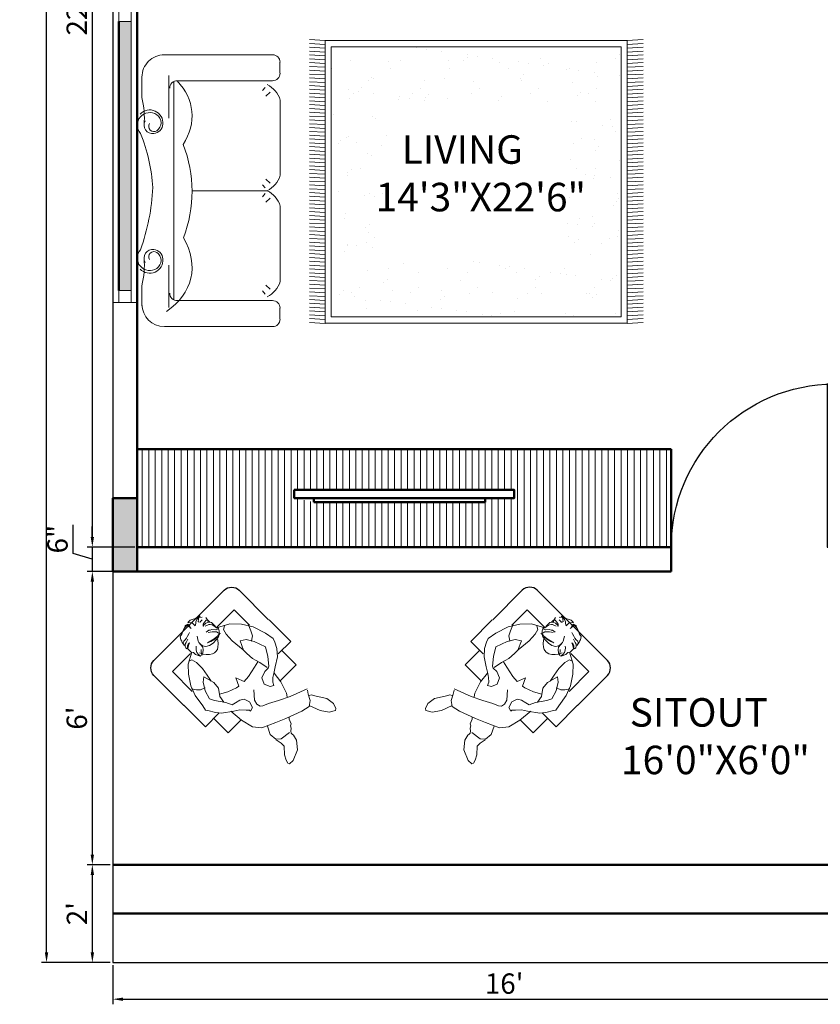
# Model space of a CAD drawing. Units: inches. Extents: x 3064 to 19385, y 846 to 15425.
# Tile 56 of 108: x 6020 to 6216, y 1462 to 1703. Entities that reach past the tile are written whole.
import ezdxf

# ---------------------------------------------------------------- set-up
doc = ezdxf.new("R2010")
doc.units = ezdxf.units.IN
for name, color, linetype, lineweight in [('A-ANNO-DIMS', 2, 'Continuous', 18), ('A-AREA-IDEN', 3, 'Continuous', 18), ('A-COLS', 1, 'Continuous', 35), ('A-DOOR', 3, 'Continuous', 25), ('A-FURN', 8, 'Continuous', 18), ('A-FURN-PATT', 252, 'Continuous', 13), ('A-GLAZ', 4, 'Continuous', 18), ('A-WALL', 7, 'Continuous', 50), ('C-PROP', 6, 'Continuous', 25)]:
    doc.layers.add(name, color=color, linetype=linetype, lineweight=lineweight)
doc.layers.add('NOITHAT', color=21, linetype='Continuous')
doc.styles.get("Standard").update_dxf_attribs({"font": 'arial.ttf'})
doc.dimstyles.new('ISO-25', dxfattribs={"dimtxt": 9, "dimasz": 2.5, "dimexe": 1.25, "dimexo": 0.625, "dimtad": 1, "dimdec": 1, "dimlunit": 3, "dimtxsty": 'Standard', "dimcen": 2.5, "dimadec": 0, "dimazin": 0, "dimtfac": 1, "dimtdec": 1, "dimtmove": 0, "dimatfit": 3, "dimfxl": 1, "dimarcsym": 0})

# ---------------------------------------------------------------- blocks, each defined once
blk = doc.blocks.new('*U2')
for p, q in [((0, 0), (0, -6)), ((40, 0), (40, -6))]:
    blk.add_line(p, q)
blk.add_lwpolyline([(0, 0), (0, 40), (1.75, 40), (1.75, 0)], close=True)
blk.add_arc((0, 0), 40, 0, 90)
blk = doc.blocks.new('carpet-9')
at = {"color": 0, "linetype": 'ByBlock'}
for p, q in [((-2.5225, -0.1423), (-2.5308, 0)), ((-2.4883, -0.1423), (-2.4966, 0)), ((-2.4541, -0.1423), (-2.4624, 0)), ((-2.4199, -0.1423), (-2.4282, 0)), ((-2.3857, -0.1423), (-2.394, 0)), ((-2.3515, -0.1423), (-2.3598, 0)), ((-2.3173, -0.1423), (-2.3256, 0)), ((-2.2831, -0.1423), (-2.2914, 0)), ((-2.2489, -0.1423), (-2.2572, 0)), ((-2.2147, -0.1423), (-2.223, 0)), ((-2.1805, -0.1423), (-2.1888, 0)), ((-2.1463, -0.1423), (-2.1546, 0)), ((-2.1121, -0.1423), (-2.1204, 0)), ((-2.0779, -0.1423), (-2.0862, 0)), ((-2.0437, -0.1423), (-2.052, 0)), ((-2.0095, -0.1423), (-2.0178, 0)), ((-1.9753, -0.1423), (-1.9836, 0)), ((-1.9411, -0.1423), (-1.9494, 0)), ((-1.9069, -0.1423), (-1.9152, 0)), ((-1.8727, -0.1423), (-1.881, 0)), ((-1.8385, -0.1423), (-1.8468, 0)), ((-1.8043, -0.1423), (-1.8126, 0)), ((-1.7701, -0.1423), (-1.7784, 0)), ((-1.7359, -0.1423), (-1.7442, 0)), ((-1.7017, -0.1423), (-1.71, 0)), ((-1.6675, -0.1423), (-1.6758, 0)), ((-1.6333, -0.1423), (-1.6416, 0)), ((-1.5991, -0.1423), (-1.6074, 0)), ((-1.5649, -0.1423), (-1.5732, 0)), ((-1.5307, -0.1423), (-1.539, 0)), ((-1.4965, -0.1423), (-1.5048, 0)), ((-1.4623, -0.1423), (-1.4706, 0)), ((-1.4281, -0.1423), (-1.4364, 0)), ((-1.3939, -0.1423), (-1.4022, 0)), ((-1.3597, -0.1423), (-1.368, 0)), ((-1.3255, -0.1423), (-1.3338, 0)), ((-1.2913, -0.1423), (-1.2996, 0)), ((-1.2571, -0.1423), (-1.2654, 0)), ((-1.2229, -0.1423), (-1.2312, 0)), ((-1.1887, -0.1423), (-1.197, 0)), ((-1.1545, -0.1423), (-1.1628, 0)), ((-1.1203, -0.1423), (-1.1286, 0)), ((-1.0861, -0.1423), (-1.0944, 0)), ((-1.0519, -0.1423), (-1.0602, 0)), ((-1.0177, -0.1423), (-1.026, 0)), ((-0.9835, -0.1423), (-0.9918, 0)), ((-0.9493, -0.1423), (-0.9576, 0)), ((-0.9151, -0.1423), (-0.9234, 0)), ((-0.8809, -0.1423), (-0.8892, 0)), ((-0.8467, -0.1423), (-0.855, 0)), ((-0.8125, -0.1423), (-0.8208, 0)), ((-0.7783, -0.1423), (-0.7866, 0)), ((-0.7441, -0.1423), (-0.7524, 0)), ((-0.7099, -0.1423), (-0.7182, 0)), ((-0.6757, -0.1423), (-0.684, 0)), ((-0.6415, -0.1423), (-0.6498, 0)), ((-0.6073, -0.1423), (-0.6156, 0)), ((-0.5731, -0.1423), (-0.5814, 0)), ((-0.5389, -0.1423), (-0.5472, 0)), ((-0.5047, -0.1423), (-0.513, 0)), ((-0.4705, -0.1423), (-0.4788, 0)), ((-0.4363, -0.1423), (-0.4446, 0)), ((-0.4021, -0.1423), (-0.4104, 0)), ((-0.3679, -0.1423), (-0.3762, 0)), ((-0.3337, -0.1423), (-0.342, 0)), ((-0.2995, -0.1423), (-0.3078, 0)), ((-0.2653, -0.1423), (-0.2736, 0)), ((-0.2311, -0.1423), (-0.2394, 0)), ((-0.1969, -0.1423), (-0.2052, 0)), ((-0.1627, -0.1423), (-0.171, 0)), ((-0.1285, -0.1423), (-0.1368, 0)), ((-0.0943, -0.1423), (-0.1026, 0)), ((-0.0601, -0.1423), (-0.0684, 0)), ((-0.0259, -0.1423), (-0.0342, 0)), ((0.0083, -0.1423), (0, 0)), ((0.0081, -0.1423), (-2.5225, -0.1423)), ((-2.5225, -0.1423), (-2.5225, -2.8423)), ((0.0081, -2.8423), (0.0081, -0.1423)), ((-0.0489, -0.1963), (-2.4655, -0.1963)), ((-2.4655, -0.1963), (-2.4655, -2.7883)), ((-2.3955, -0.2124), (-2.3955, -0.2124)), ((-2.3654, -0.2435), (-2.3654, -0.2435)), ((-2.2062, -0.2078), (-2.2062, -0.2078)), ((-1.7121, -0.2501), (-1.7121, -0.2501)), ((-1.4511, -0.2068), (-1.4511, -0.2068)), ((-1.1533, -0.2312), (-1.1533, -0.2312)), ((-1.1079, -0.2175), (-1.1079, -0.2175)), ((-1.0792, -0.2355), (-1.0792, -0.2355)), ((-0.8244, -0.2203), (-0.8244, -0.2203)), ((-0.7647, -0.2281), (-0.7647, -0.2281)), ((-0.4215, -0.2387), (-0.4215, -0.2387)), ((-0.0783, -0.2494), (-0.0783, -0.2494)), ((-0.0489, -2.7883), (-0.0489, -0.1963)), ((-1.8205, -0.2931), (-1.8205, -0.2931)), ((-1.7544, -0.2756), (-1.7544, -0.2756)), ((-1.2958, -0.294), (-1.2958, -0.294)), ((-1.0491, -0.2666), (-1.0491, -0.2666)), ((-0.7551, -0.2963), (-0.7551, -0.2963)), ((-0.3958, -0.2731), (-0.3958, -0.2731)), ((-0.3726, -0.2881), (-0.3726, -0.2881)), ((-2.3219, -0.4132), (-2.3219, -0.4132)), ((-2.2381, -0.437), (-2.2381, -0.437)), ((-2.203, -0.4115), (-2.203, -0.4115)), ((-2.0942, -0.413), (-2.0942, -0.413)), ((-1.9787, -0.4238), (-1.9787, -0.4238)), ((-1.7666, -0.3634), (-1.7666, -0.3634)), ((-1.6355, -0.4344), (-1.6355, -0.4344)), ((-1.5701, -0.3969), (-1.5701, -0.3969)), ((-1.54, -0.428), (-1.54, -0.428)), ((-1.3744, -0.4294), (-1.3744, -0.4294)), ((-1.3149, -0.4312), (-1.3149, -0.4312)), ((-0.8867, -0.4345), (-0.8867, -0.4345)), ((-0.7072, -0.3675), (-0.7072, -0.3675)), ((-0.3848, -0.3759), (-0.3848, -0.3759)), ((-0.3091, -0.4326), (-0.3091, -0.4326)), ((-0.2538, -0.4199), (-0.2538, -0.4199)), ((-2.0464, -0.4841), (-2.0464, -0.4841)), ((-1.3271, -0.519), (-1.3271, -0.519)), ((-1.2923, -0.4451), (-1.2923, -0.4451)), ((-0.949, -0.4557), (-0.949, -0.4557)), ((-0.8562, -0.4496), (-0.8562, -0.4496)), ((-0.6058, -0.4663), (-0.6058, -0.4663)), ((-0.2626, -0.477), (-0.2626, -0.477)), ((-0.2612, -0.5038), (-0.2612, -0.5038)), ((-0.2237, -0.451), (-0.2237, -0.451)), ((-2.2571, -0.5742), (-2.2571, -0.5742)), ((-2.061, -0.5583), (-2.061, -0.5583)), ((-2.0309, -0.5894), (-2.0309, -0.5894)), ((-1.7985, -0.5926), (-1.7985, -0.5926)), ((-1.6482, -0.5493), (-1.6482, -0.5493)), ((-1.3776, -0.5959), (-1.3776, -0.5959)), ((-0.9284, -0.5657), (-0.9284, -0.5657)), ((-0.8753, -0.5867), (-0.8753, -0.5867)), ((-0.7447, -0.5813), (-0.7447, -0.5813)), ((-0.7146, -0.6124), (-0.7146, -0.6124)), ((-0.4167, -0.6051), (-0.4167, -0.6051)), ((-2.2693, -0.6621), (-2.2693, -0.6621)), ((-2.2675, -0.6823), (-2.2675, -0.6823)), ((-2.1435, -0.6273), (-2.1435, -0.6273)), ((-1.8003, -0.6379), (-1.8003, -0.6379)), ((-1.6003, -0.6204), (-1.6003, -0.6204)), ((-1.4571, -0.6486), (-1.4571, -0.6486)), ((-1.2021, -0.6856), (-1.2021, -0.6856)), ((-1.1139, -0.6592), (-1.1139, -0.6592)), ((-0.8875, -0.6746), (-0.8875, -0.6746)), ((-0.7706, -0.6698), (-0.7706, -0.6698)), ((-0.4823, -0.702), (-0.4823, -0.702)), ((-0.4274, -0.6805), (-0.4274, -0.6805)), ((-0.0842, -0.6911), (-0.0842, -0.6911)), ((-0.0613, -0.619), (-0.0613, -0.619)), ((-0.4357, -0.7423), (-0.4357, -0.7423)), ((-2.3197, -0.8449), (-2.3197, -0.8449)), ((-1.9765, -0.8555), (-1.9765, -0.8555)), ((-0.4479, -0.8302), (-0.4479, -0.8302)), ((-2.3593, -0.9188), (-2.3593, -0.9188)), ((-2.3012, -0.8913), (-2.3012, -0.8913)), ((-2.0952, -0.9385), (-2.0952, -0.9385)), ((-0.4101, -0.9272), (-0.4101, -0.9272)), ((-0.3801, -0.9583), (-0.3801, -0.9583)), ((-0.3101, -0.9581), (-0.3101, -0.9581)), ((-0.2604, -0.9086), (-0.2604, -0.9086)), ((-2.3203, -1.0285), (-2.3203, -1.0285)), ((-2.0474, -1.0097), (-2.0474, -1.0097)), ((-0.2622, -1.0293), (-0.2622, -1.0293)), ((-2.3325, -1.1163), (-2.3325, -1.1163)), ((-2.2173, -1.0656), (-2.2173, -1.0656)), ((-2.1872, -1.0967), (-2.1872, -1.0967)), ((-2.1608, -1.0831), (-2.1608, -1.0831)), ((-0.4798, -1.0594), (-0.4798, -1.0594)), ((-0.4448, -1.1362), (-0.4448, -1.1362)), ((-0.2176, -1.1263), (-0.2176, -1.1263)), ((-2.2685, -1.2078), (-2.2685, -1.2078)), ((-0.4989, -1.1966), (-0.4989, -1.1966)), ((-0.4833, -1.2275), (-0.4833, -1.2275)), ((-0.1015, -1.1469), (-0.1015, -1.1469)), ((-2.3257, -1.2866), (-2.3257, -1.2866)), ((-2.0248, -1.2646), (-2.0248, -1.2646)), ((-1.9824, -1.2972), (-1.9824, -1.2972)), ((-0.5111, -1.2844), (-0.5111, -1.2844)), ((-0.0756, -1.2731), (-0.0756, -1.2731)), ((-2.3643, -1.3455), (-2.3643, -1.3455)), ((-0.2664, -1.3504), (-0.2664, -1.3504)), ((-0.0593, -1.3522), (-0.0593, -1.3522)), ((-2.3834, -1.4827), (-2.3834, -1.4827)), ((-2.0963, -1.464), (-2.0963, -1.464)), ((-0.5364, -1.4656), (-0.5364, -1.4656)), ((-0.3111, -1.4836), (-0.3111, -1.4836)), ((-0.0715, -1.44), (-0.0715, -1.44)), ((-2.3956, -1.5705), (-2.3956, -1.5705)), ((-2.3737, -1.5729), (-2.3737, -1.5729)), ((-2.1587, -1.5148), (-2.1587, -1.5148)), ((-2.0484, -1.5352), (-2.0484, -1.5352)), ((-0.5429, -1.5136), (-0.5429, -1.5136)), ((-0.4426, -1.5679), (-0.4426, -1.5679)), ((-0.2632, -1.5548), (-0.2632, -1.5548)), ((-0.0994, -1.5785), (-0.0994, -1.5785)), ((-2.3436, -1.604), (-2.3436, -1.604)), ((-0.3739, -1.6336), (-0.3739, -1.6336)), ((-0.1033, -1.6692), (-0.1033, -1.6692)), ((-2.343, -1.7423), (-2.343, -1.7423)), ((-2.2695, -1.7333), (-2.2695, -1.7333)), ((-1.9998, -1.753), (-1.9998, -1.753)), ((-0.4843, -1.753), (-0.4843, -1.753)), ((-2.4274, -1.7997), (-2.4274, -1.7997)), ((-2.1811, -1.7719), (-2.1811, -1.7719)), ((-0.2837, -1.8061), (-0.2837, -1.8061)), ((-0.2319, -1.7804), (-0.2319, -1.7804)), ((-0.2018, -1.8115), (-0.2018, -1.8115)), ((-0.1224, -1.8064), (-0.1224, -1.8064)), ((-2.4465, -1.9369), (-2.4465, -1.9369)), ((-2.0391, -1.9187), (-2.0391, -1.9187)), ((-0.1346, -1.8942), (-0.1346, -1.8942)), ((-2.4587, -2.0248), (-2.4587, -2.0248)), ((-2.1646, -1.9565), (-2.1646, -1.9565)), ((-2.0973, -1.9895), (-2.0973, -1.9895)), ((-2.009, -1.9498), (-2.009, -1.9498)), ((-1.9879, -1.9553), (-1.9879, -1.9553)), ((-0.4485, -2.0096), (-0.4485, -2.0096)), ((-0.3121, -2.0092), (-0.3121, -2.0092)), ((-0.1053, -2.0203), (-0.1053, -2.0203)), ((-2.0494, -2.0607), (-2.0494, -2.0607)), ((-2.0069, -2.0925), (-2.0069, -2.0925)), ((-0.2642, -2.0803), (-0.2642, -2.0803)), ((-2.3408, -2.174), (-2.3408, -2.174)), ((-2.0191, -2.1804), (-2.0191, -2.1804)), ((-1.9976, -2.1847), (-1.9976, -2.1847)), ((-0.5303, -2.1409), (-0.5303, -2.1409)), ((-0.1665, -2.1234), (-0.1665, -2.1234)), ((-2.3374, -2.2792), (-2.3374, -2.2792)), ((-2.2705, -2.2589), (-2.2705, -2.2589)), ((-0.4854, -2.2785), (-0.4854, -2.2785)), ((-0.3883, -2.2877), (-0.3883, -2.2877)), ((-0.2815, -2.2378), (-0.2815, -2.2378)), ((-0.1855, -2.2606), (-0.1855, -2.2606)), ((-1.6745, -2.2957), (-1.6745, -2.2957)), ((-1.5796, -2.3359), (-1.5796, -2.3359)), ((-1.1573, -2.3333), (-1.1573, -2.3333)), ((-1.0211, -2.3023), (-1.0211, -2.3023)), ((-0.3582, -2.3188), (-0.3582, -2.3188)), ((-0.1977, -2.3485), (-0.1977, -2.3485)), ((-2.1954, -2.426), (-2.1954, -2.426)), ((-2.1819, -2.4122), (-2.1819, -2.4122)), ((-2.1654, -2.4571), (-2.1654, -2.4571)), ((-2.051, -2.4096), (-2.051, -2.4096)), ((-1.8387, -2.4229), (-1.8387, -2.4229)), ((-1.8245, -2.3951), (-1.8245, -2.3951)), ((-1.512, -2.4637), (-1.512, -2.4637)), ((-1.4955, -2.4335), (-1.4955, -2.4335)), ((-1.1523, -2.4441), (-1.1523, -2.4441)), ((-1.1278, -2.4037), (-1.1278, -2.4037)), ((-0.8791, -2.4491), (-0.8791, -2.4491)), ((-0.8091, -2.4548), (-0.8091, -2.4548)), ((-0.7591, -2.3984), (-0.7591, -2.3984)), ((-0.6692, -2.4221), (-0.6692, -2.4221)), ((-0.4659, -2.4654), (-0.4659, -2.4654)), ((-2.0983, -2.515), (-2.0983, -2.515)), ((-2.0701, -2.5468), (-2.0701, -2.5468)), ((-1.3785, -2.5314), (-1.3785, -2.5314)), ((-1.14, -2.4915), (-1.14, -2.4915)), ((-0.8491, -2.4802), (-0.8491, -2.4802)), ((-0.7113, -2.4695), (-0.7113, -2.4695)), ((-0.3131, -2.5347), (-0.3131, -2.5347)), ((-0.1957, -2.4867), (-0.1957, -2.4867)), ((-0.1226, -2.476), (-0.1226, -2.476)), ((-2.3468, -2.6157), (-2.3468, -2.6157)), ((-2.0823, -2.6346), (-2.0823, -2.6346)), ((-2.0504, -2.5862), (-2.0504, -2.5862)), ((-2.0035, -2.6264), (-2.0035, -2.6264)), ((-2.0029, -2.6251), (-2.0029, -2.6251)), ((-1.6603, -2.637), (-1.6603, -2.637)), ((-1.6114, -2.5652), (-1.6114, -2.5652)), ((-1.37, -2.6105), (-1.37, -2.6105)), ((-1.3399, -2.6416), (-1.3399, -2.6416)), ((-0.6882, -2.5593), (-0.6882, -2.5593)), ((-0.2652, -2.6058), (-0.2652, -2.6058)), ((-0.2296, -2.5777), (-0.2296, -2.5777)), ((-0.0537, -2.6335), (-0.0537, -2.6335)), ((-1.6522, -2.6513), (-1.6522, -2.6513)), ((-1.6305, -2.7023), (-1.6305, -2.7023)), ((-1.6044, -2.7225), (-1.6044, -2.7225)), ((-1.3171, -2.6476), (-1.3171, -2.6476)), ((-1.1719, -2.7207), (-1.1719, -2.7207)), ((-0.9739, -2.6583), (-0.9739, -2.6583)), ((-0.9324, -2.6677), (-0.9324, -2.6677)), ((-0.7004, -2.6471), (-0.7004, -2.6471)), ((-0.6866, -2.6481), (-0.6866, -2.6481)), ((-0.6307, -2.6689), (-0.6307, -2.6689)), ((-0.2875, -2.6795), (-0.2875, -2.6795)), ((-0.2487, -2.7149), (-0.2487, -2.7149)), ((-2.4655, -2.7883), (-0.0489, -2.7883)), ((-2.2715, -2.7844), (-2.2715, -2.7844)), ((-1.8609, -2.7719), (-1.8609, -2.7719)), ((-1.2062, -2.7876), (-1.2062, -2.7876)), ((-2.5225, -2.8423), (-2.5308, -2.9845)), ((-2.5225, -2.8423), (0.0081, -2.8423)), ((-2.4883, -2.8423), (-2.4966, -2.9845)), ((-2.4541, -2.8423), (-2.4624, -2.9845)), ((-2.4199, -2.8423), (-2.4282, -2.9845)), ((-2.3857, -2.8423), (-2.394, -2.9845)), ((-2.3515, -2.8423), (-2.3598, -2.9845)), ((-2.3173, -2.8423), (-2.3256, -2.9845)), ((-2.2831, -2.8423), (-2.2914, -2.9845)), ((-2.2489, -2.8423), (-2.2572, -2.9845)), ((-2.2147, -2.8423), (-2.223, -2.9845)), ((-2.1805, -2.8423), (-2.1888, -2.9845)), ((-2.1463, -2.8423), (-2.1546, -2.9845)), ((-2.1121, -2.8423), (-2.1204, -2.9845)), ((-2.0779, -2.8423), (-2.0862, -2.9845)), ((-2.0437, -2.8423), (-2.052, -2.9845)), ((-2.0095, -2.8423), (-2.0178, -2.9845)), ((-1.9753, -2.8423), (-1.9836, -2.9845)), ((-1.9411, -2.8423), (-1.9494, -2.9845)), ((-1.9069, -2.8423), (-1.9152, -2.9845)), ((-1.8727, -2.8423), (-1.881, -2.9845)), ((-1.8385, -2.8423), (-1.8468, -2.9845)), ((-1.8043, -2.8423), (-1.8126, -2.9845)), ((-1.7701, -2.8423), (-1.7784, -2.9845)), ((-1.7359, -2.8423), (-1.7442, -2.9845)), ((-1.7017, -2.8423), (-1.71, -2.9845)), ((-1.6675, -2.8423), (-1.6758, -2.9845)), ((-1.6333, -2.8423), (-1.6416, -2.9845)), ((-1.5991, -2.8423), (-1.6074, -2.9845)), ((-1.5649, -2.8423), (-1.5732, -2.9845)), ((-1.5307, -2.8423), (-1.539, -2.9845)), ((-1.4965, -2.8423), (-1.5048, -2.9845)), ((-1.4623, -2.8423), (-1.4706, -2.9845)), ((-1.4281, -2.8423), (-1.4364, -2.9845)), ((-1.3939, -2.8423), (-1.4022, -2.9845)), ((-1.3597, -2.8423), (-1.368, -2.9845)), ((-1.3255, -2.8423), (-1.3338, -2.9845)), ((-1.2913, -2.8423), (-1.2996, -2.9845)), ((-1.2571, -2.8423), (-1.2654, -2.9845)), ((-1.2229, -2.8423), (-1.2312, -2.9845)), ((-1.1887, -2.8423), (-1.197, -2.9845)), ((-1.1545, -2.8423), (-1.1628, -2.9845)), ((-1.1203, -2.8423), (-1.1286, -2.9845)), ((-1.0861, -2.8423), (-1.0944, -2.9845)), ((-1.0519, -2.8423), (-1.0602, -2.9845)), ((-1.0177, -2.8423), (-1.026, -2.9845)), ((-0.9835, -2.8423), (-0.9918, -2.9845)), ((-0.9493, -2.8423), (-0.9576, -2.9845)), ((-0.9151, -2.8423), (-0.9234, -2.9845)), ((-0.8809, -2.8423), (-0.8892, -2.9845)), ((-0.8467, -2.8423), (-0.855, -2.9845)), ((-0.8125, -2.8423), (-0.8208, -2.9845)), ((-0.7783, -2.8423), (-0.7866, -2.9845)), ((-0.7441, -2.8423), (-0.7524, -2.9845)), ((-0.7099, -2.8423), (-0.7182, -2.9845)), ((-0.6757, -2.8423), (-0.684, -2.9845)), ((-0.6415, -2.8423), (-0.6498, -2.9845)), ((-0.6073, -2.8423), (-0.6156, -2.9845)), ((-0.5731, -2.8423), (-0.5814, -2.9845)), ((-0.5389, -2.8423), (-0.5472, -2.9845)), ((-0.5047, -2.8423), (-0.513, -2.9845)), ((-0.4705, -2.8423), (-0.4788, -2.9845)), ((-0.4363, -2.8423), (-0.4446, -2.9845)), ((-0.4021, -2.8423), (-0.4104, -2.9845)), ((-0.3679, -2.8423), (-0.3762, -2.9845)), ((-0.3337, -2.8423), (-0.342, -2.9845)), ((-0.2995, -2.8423), (-0.3078, -2.9845)), ((-0.2653, -2.8423), (-0.2736, -2.9845)), ((-0.2311, -2.8423), (-0.2394, -2.9845)), ((-0.1969, -2.8423), (-0.2052, -2.9845)), ((-0.1627, -2.8423), (-0.171, -2.9845)), ((-0.1285, -2.8423), (-0.1368, -2.9845)), ((-0.0943, -2.8423), (-0.1026, -2.9845)), ((-0.0601, -2.8423), (-0.0684, -2.9845)), ((-0.0259, -2.8423), (-0.0342, -2.9845)), ((0.0083, -2.8423), (0, -2.9845))]:
    blk.add_line(p, q, dxfattribs=at)
blk = doc.blocks.new('sofa-33')
at = {"color": 0, "linetype": 'ByBlock'}
for p, q in [((-0.026, 0.9238), (-0.1, 0.9238)), ((0.657, 0.9252), (0.1531, 0.9252)), ((0.8633, 0.9252), (1.3671, 0.9252)), ((1.6203, 0.9238), (1.5463, 0.9238)), ((-0.15, 0.15), (-0.15, 0.8738)), ((0.024, 0.2361), (0.024, 0.8738)), ((0.1006, 0.8574), (0.1265, 0.8286)), ((0.7096, 0.8574), (0.6837, 0.8286)), ((0.8107, 0.8574), (0.8366, 0.8286)), ((1.4197, 0.8574), (1.3938, 0.8286)), ((1.4963, 0.2361), (1.4963, 0.8738)), ((1.6703, 0.15), (1.6703, 0.8738)), ((0.05, 0.8375), (0.05, 0.8379)), ((0.0903, 0.8062), (0.0682, 0.8242)), ((0.7199, 0.8062), (0.742, 0.8242)), ((0.7602, 0.8375), (0.7601, 0.8379)), ((0.7601, 0.8375), (0.7601, 0.8379)), ((0.7602, 0.8375), (0.7602, 0.3356)), ((0.8004, 0.8062), (0.7783, 0.8242)), ((1.43, 0.8062), (1.4521, 0.8242)), ((1.4702, 0.8375), (1.4703, 0.8379)), ((1.4702, 0.8375), (1.4703, 0.8379)), ((0.0289, 0.2145), (1.4914, 0.2145)), ((-0.01, 0.1801), (0.2738, 0.1801)), ((1.5422, 0.1801), (1.2585, 0.1801)), ((0, 0), (0.1356, 0)), ((1.5322, 0), (1.3966, 0))]:
    blk.add_line(p, q, dxfattribs=at)
at = {"color": 0, "linetype": 'ByBlock', "extrusion": (0, 0, -1)}
for centre, major_axis, ratio, start_param, end_param in [((-0.1, 0.8738), (0.0354, 0.0354), 1, 3.926992, 5.497787), ((-0.026, 0.8738), (-0.0354, 0.0354), 1, 0.785398, 2.356196), ((0.1997, 0.7661), (0.1173, 0.1173), 1, 4.372209, 5.213218), ((0.6105, 0.7661), (0.1173, 0.1173), 1, -0.500829, 0.34018), ((0.9098, 0.7661), (0.1173, 0.1173), 1, 4.372209, 5.213218), ((1.3206, 0.7661), (-0.1173, 0.1173), 1, 1.069968, 1.910976), ((1.5463, 0.8738), (-0.0354, 0.0354), 1, 5.497786, 7.068583), ((1.6203, 0.8738), (0.0354, 0.0354), 1, -0.785398, 0.785398), ((0.3234, -0.6657), (-0.0931, 0.9998), 0.551284, -0.397889, 0.397889), ((0.7664, -0.6685), (-0.0034, 1.0041), 0.922365, -0.343589, 0.343589), ((1.147, -0.5336), (0.1998, 0.8608), 0.59532, -0.502747, 0.502747), ((0.074, 0.2361), (-0.0354, 0.0354), 1, 3.926991, 5.497788), ((1.4463, 0.2361), (0.0354, 0.0354), 1, 0.785397, 2.356194), ((0, 0.15), (0.1061, 0.1061), 1, 2.356194, 3.926992), ((0.3076, 0.0525), (-0.0624, 0.0624), 1, 4.675944, 7.152385), ((0.3092, 0.0712), (0.0491, 0.0491), 1, -0.701597, 0.659711), ((1.223, 0.0712), (-0.0491, 0.0491), 1, 5.623477, 6.984784), ((1.2246, 0.0525), (-0.0624, 0.0624), 1, 0.701599, 3.17804), ((1.5203, 0.15), (0.1061, 0.1061), 1, 0.785398, 2.356194), ((0.3208, 0.0524), (-0.059, 0.059), 1, 3.186406, 6.094039), ((0.3052, 0.0629), (-0.0458, 0.0458), 1, 6.094039, 8.043134), ((0.3201, 0.0726), (-0.0414, 0.0414), 1, 2.230507, 4.423483), ((0.3301, 0.0798), (0.0245, 0.0245), 1, 0.189152, 2.952444), ((0.8779, -1.3822), (-0.3228, 1.4289), 0.878591, -0.144977, 0.144977), ((0.6669, -1.3904), (1.0359, 1.0359), 1, 5.547613, 5.837566), ((1.2122, 0.0726), (-0.0414, 0.0414), 1, 3.430501, 5.623477), ((1.2115, 0.0524), (0.059, 0.059), 1, 0.189149, 3.096782), ((1.2022, 0.0798), (0.0245, 0.0245), 1, 1.759947, 4.52324), ((1.227, 0.0629), (0.0458, 0.0458), 1, 4.52324, 6.472335), ((0.2824, -0.6613), (-0.479, 0.479), 1, 0.566947, 0.842011), ((1.2498, -0.6613), (0.479, 0.479), 1, 5.441177, 5.716241)]:
    blk.add_ellipse(centre, major_axis=major_axis, ratio=ratio, start_param=start_param, end_param=end_param, dxfattribs=at)
blk = doc.blocks.new('A$C48E80792')
for p, q in [((208.1, 777.4), (217.7, 791.8)), ((217.7, 791.8), (230.8, 792.5)), ((230.8, 792.5), (252, 804.1)), ((252, 804.1), (267.8, 807.6)), ((253.5, 801.9), (261.1, 805.7)), ((261.1, 805.7), (274.4, 805.7)), ((267.8, 807.6), (270.5, 811.7)), ((284, 805.7), (270.6, 811.4)), ((274.4, 805.7), (278.3, 805.7)), ((278.3, 805.7), (278.3, 798.1)), ((278.3, 798.1), (280.2, 788.5)), ((280.2, 786.6), (284, 794.3)), ((284, 794.3), (284, 805.7)), ((289.7, 811.4), (305.5, 811.7)), ((289.7, 811.4), (303, 796.2)), ((303, 796.2), (303, 779)), ((305.5, 811.7), (317.9, 805.5)), ((317.9, 805.5), (328.1, 800)), ((318.3, 788.5), (329.8, 792.4)), ((328.1, 800), (343.9, 798)), ((329.8, 792.4), (343.1, 794.3)), ((343.1, 792.4), (335.5, 786.6)), ((343.1, 794.3), (352.6, 794.3)), ((352.6, 792.4), (343.1, 792.4)), ((343.9, 798), (352.1, 795.9)), ((343.9, 790.4), (354.9, 782.2)), ((202, 746.6), (204.7, 764.4)), ((202, 746.6), (205.8, 759.9)), ((202, 742.8), (207.7, 748.5)), ((204.7, 764.4), (207.4, 769.9)), ((205.8, 759.9), (213.4, 763.8)), ((207.4, 769.9), (208.1, 777.4)), ((207.7, 748.5), (217.2, 750.4)), ((213.4, 763.8), (222.9, 763.8)), ((217.2, 750.4), (226.8, 754.2)), ((222.9, 763.8), (232.5, 763.8)), ((226.8, 754.2), (234.4, 756.1)), ((232.5, 763.8), (236.3, 765.7)), ((236.3, 765.7), (242, 767.6)), ((242, 767.6), (255.4, 771.4)), ((255.4, 771.4), (261.1, 773.3)), ((280.2, 788.5), (280.2, 780.9)), ((280.2, 780.9), (280.2, 786.6)), ((303, 777.1), (312.6, 782.8)), ((303, 779), (303, 777.1)), ((312.6, 782.8), (318.3, 788.5)), ((335.5, 786.6), (327.8, 780.9)), ((327.8, 780.9), (327.8, 775.2)), ((327.8, 748.5), (335.5, 756.1)), ((329.8, 748.5), (327.8, 748.5)), ((329.8, 771.4), (335.5, 773.3)), ((335.5, 750.4), (329.8, 748.5)), ((335.5, 773.3), (346.9, 773.3)), ((335.5, 756.1), (346.9, 758)), ((337.4, 750.4), (335.5, 750.4)), ((341.2, 750.4), (337.4, 750.4)), ((346.9, 750.4), (341.2, 750.4)), ((346.9, 758), (358.4, 758)), ((354.5, 746.6), (346.9, 750.4)), ((362.2, 742.8), (354.5, 746.6)), ((362.2, 750.4), (356.5, 746.6)), ((358.4, 758), (362.2, 756.1)), ((366, 769.5), (362.2, 750.4)), ((362.2, 756.1), (364.1, 750.4)), ((364.1, 750.4), (364.1, 742.8)), ((204, 699.4), (151.7, 671.2)), ((198.1, 735.2), (202, 742.8)), ((198.1, 727.5), (198.1, 735.2)), ((202, 727.5), (200.1, 725.6)), ((211.5, 737.1), (202, 727.5)), ((202, 723.7), (209.6, 729.4)), ((202, 716.1), (202, 723.7)), ((202, 706.6), (202, 716.1)), ((202, 702.8), (202, 706.6)), ((207.7, 693.2), (202, 702.8)), ((209.6, 729.4), (219.1, 735.2)), ((219.1, 739), (211.5, 737.1)), ((226.8, 739), (219.1, 739)), ((219.1, 735.2), (226.8, 739)), ((224.8, 691.3), (232.5, 700.8)), ((226.8, 739), (226.8, 739)), ((232.5, 700.8), (238.2, 704.7)), ((259.2, 708.5), (257.3, 679.9)), ((260.3, 708.9), (259.6, 699.3)), ((259.6, 699.3), (261.6, 685.6)), ((261.6, 715.7), (260.3, 708.9)), ((274, 735.6), (261.6, 715.7)), ((318.3, 718), (333.6, 716.1)), ((331.7, 706.6), (324, 710.4)), ((339.3, 700.8), (331.7, 706.6)), ((333.6, 716.1), (339.3, 712.3)), ((352.6, 735.2), (335.5, 742.8)), ((339.3, 712.3), (346.9, 708.5)), ((346.9, 693.2), (339.3, 700.8)), ((346.9, 708.5), (358.4, 695.1)), ((356.5, 731.3), (352.6, 735.2)), ((362.2, 723.7), (356.5, 731.3)), ((367.9, 733.3), (362.2, 742.8)), ((364.1, 718), (362.2, 723.7)), ((364.1, 742.8), (364.1, 739)), ((366, 706.6), (364.1, 718)), ((367.9, 698.9), (366, 706.6)), ((366.5, 698.9), (425.1, 668)), ((367.9, 706.6), (367.9, 733.3)), ((371.7, 691.3), (367.9, 698.9)), ((151.7, 671.2), (119.2, 637.1)), ((165.1, 679.5), (178.4, 675)), ((178.4, 675), (185.1, 650.5)), ((207.7, 679.9), (207.7, 693.2)), ((219.1, 658.9), (207.7, 679.9)), ((219.1, 681.8), (224.8, 691.3)), ((219.1, 670.3), (219.1, 681.8)), ((221, 657), (219.1, 670.3)), ((226.8, 655.1), (232.5, 664.6)), ((232.5, 657), (226.8, 655.1)), ((227.3, 673.2), (235.6, 655.4)), ((232.5, 664.6), (236.3, 670.3)), ((238.2, 660.8), (232.5, 657)), ((235.6, 655.4), (243.8, 644.4)), ((236.3, 670.3), (243.9, 678)), ((249.6, 670.3), (238.2, 660.8)), ((257.3, 679.9), (249.6, 670.3)), ((261.6, 685.6), (269.2, 671.8)), ((269.2, 671.8), (285.6, 662.9)), ((285.6, 662.9), (304.8, 659.5)), ((302.1, 672.5), (287, 679.4)), ((287, 679.4), (304.8, 673.9)), ((323.3, 667), (302.1, 672.5)), ((304.8, 673.9), (323.3, 670.5)), ((304.8, 659.5), (326.8, 659.5)), ((319.2, 640.3), (330.9, 654)), ((323.3, 670.5), (345.3, 668.4)), ((337.7, 666.4), (323.3, 667)), ((326.8, 659.5), (340.5, 661.6)), ((330.9, 654), (334, 660.6)), ((356.3, 669.8), (337.7, 666.4)), ((340.5, 661.6), (348.7, 664.3)), ((345.3, 668.4), (356.3, 668.4)), ((354.5, 685.6), (346.9, 693.2)), ((348.7, 664.3), (352.1, 667.7)), ((352.1, 667.7), (356.3, 669.8)), ((356.5, 676.1), (354.5, 685.6)), ((356.3, 668.4), (367.2, 680.1)), ((356.3, 668.4), (358.3, 669.8)), ((362.2, 666.5), (356.5, 676.1)), ((358.4, 695.1), (360.3, 693.2)), ((360.3, 693.2), (366, 691.3)), ((366, 691.3), (369.8, 689.4)), ((367.2, 680.1), (370.7, 689)), ((369.8, 689.4), (371.7, 689.4)), ((371.7, 689.4), (371.7, 691.3)), ((371.7, 689.4), (371.7, 689.4)), ((385.6, 670.5), (378.9, 646.1)), ((401.2, 679.5), (385.6, 670.5)), ((425.1, 668), (462.5, 627.3)), ((119.2, 637.1), (88.2, 591.5)), ((185.1, 610.4), (178.4, 572.6)), ((185.1, 650.5), (185.1, 610.4)), ((243.8, 644.4), (254.8, 633.5)), ((254.8, 633.5), (267.8, 625.9)), ((267.8, 625.9), (276.7, 622.5)), ((276.7, 622.5), (283.6, 621.8)), ((283.6, 621.8), (298, 623.9)), ((298, 623.9), (307.6, 630.7)), ((307.6, 630.7), (319.2, 640.3)), ((378.9, 646.1), (376.7, 603.8)), ((462.5, 627.3), (493.4, 580.1)), ((485.8, 606), (472.4, 574.8)), ((88.2, 591.5), (70.3, 544.3)), ((80.4, 579.3), (93.8, 559.2)), ((93.8, 559.2), (107.1, 545.9)), ((119.2, 526.5), (141.9, 562.2)), ((141.9, 562.2), (161.5, 576.9)), ((161.5, 576.9), (175.7, 525.7)), ((178.4, 572.6), (171.7, 539.2)), ((376.7, 603.8), (383.3, 537)), ((402.3, 576.9), (383.3, 535)), ((426.7, 560.6), (402.3, 576.9)), ((447.9, 528.1), (426.7, 560.6)), ((472.4, 574.8), (461.3, 552.6)), ((493.4, 580.1), (513, 518.3)), ((70.3, 544.3), (60.6, 484.2)), ((106.8, 485.6), (119.2, 526.5)), ((107.1, 545.9), (125, 539.2)), ((125, 539.2), (129.4, 537)), ((175.7, 525.7), (172, 490.5)), ((383.3, 535), (383.3, 512.7)), ((383.3, 512.7), (385.2, 475.7)), ((461.3, 552.6), (441.3, 539.2)), ((441.3, 539.2), (441.3, 537)), ((467.4, 472.8), (447.9, 528.1)), ((513, 518.3), (521.1, 474.4)), ((60.6, 484.2), (55.7, 461.4)), ((117.5, 463), (106.8, 485.6)), ((172, 490.5), (149.7, 459)), ((156.1, 468), (191.8, 447.9)), ((247.5, 430.1), (265.3, 468)), ((265.3, 468), (276.4, 439)), ((385.2, 475.7), (396.3, 438.6)), ((443, 432.1), (467.4, 472.8)), ((521.1, 474.4), (514.6, 456.5)), ((55.7, 461.4), (62.2, 451.6)), ((62.2, 451.6), (81.7, 419.1)), ((81.7, 419.1), (99.6, 398)), ((149.1, 418.9), (117.5, 463)), ((149.7, 459), (143.7, 426.5)), ((163.7, 389.7), (149.1, 418.9)), ((191.8, 447.9), (234.1, 432.3)), ((234.1, 432.3), (247.5, 430.1)), ((276.4, 439), (280.9, 427.9)), ((280.9, 427.9), (312.1, 430.1)), ((312.1, 430.1), (363.3, 441.2)), ((363.3, 441.2), (392.3, 447.9)), ((396.3, 438.6), (403.7, 397.8)), ((413.7, 396.3), (443, 432.1)), ((499.9, 428.9), (473.9, 399.6)), ((514.6, 456.5), (499.9, 428.9)), ((99.6, 398), (147.5, 363.6)), ((136.8, 373.8), (142.3, 307)), ((180, 384.8), (163.7, 389.7)), ((204.4, 379.9), (180, 384.8)), ((222.3, 368.5), (204.4, 379.9)), ((338.8, 352.4), (351.9, 380.1)), ((351.9, 380.1), (382.8, 393.1)), ((382.8, 393.1), (405.6, 391.5)), ((405.6, 391.5), (413.7, 396.3)), ((433.2, 373.6), (405.6, 355.7)), ((473.9, 399.6), (433.2, 373.6)), ((147.5, 363.6), (171.9, 347.4)), ((171.9, 347.4), (191.4, 326.2)), ((191.4, 326.2), (202.8, 314.8)), ((230.5, 340.9), (222.3, 368.5)), ((222.3, 313.2), (230.5, 340.9)), ((252.6, 331.3), (247.7, 310.1)), ((285.1, 367.1), (252.6, 331.3)), ((350.2, 324.8), (338.8, 352.4)), ((373, 329.7), (366.5, 315)), ((389.3, 345.9), (373, 329.7)), ((405.6, 355.7), (389.3, 345.9)), ((407.4, 355.2), (401.9, 303.3)), ((142.3, 307), (157.1, 247.7)), ((202.8, 314.8), (202.8, 306.7)), ((202.8, 306.7), (222.3, 313.2)), ((247.7, 310.1), (251, 292.3)), ((251, 292.3), (262.4, 284.1)), ((262.4, 284.1), (288.4, 272.7)), ((366.5, 315), (350.2, 324.8)), ((401.9, 303.3), (383.3, 247.7)), ((157.1, 247.7), (185, 214.4)), ((288.4, 272.7), (332.3, 250)), ((332.3, 250), (384.4, 223.9)), ((383.3, 247.7), (372.2, 232.9)), ((185, 214.4), (249.8, 184.7)), ((209.1, 201.4), (190.5, 164.4)), ((384.4, 223.9), (466, 193.4)), ((452.7, 171.9), (462.5, 188.2)), ((190.5, 164.4), (194.2, 129.2)), ((249.8, 184.7), (296.2, 164.4)), ((295.8, 130.1), (305.5, 151.4)), ((296.2, 164.4), (374.1, 136.6)), ((305.5, 151.4), (311, 157)), ((413, 127.3), (437.1, 144)), ((437.1, 144), (452.7, 171.9)), ((461.2, 158.8), (450.1, 164.4)), ((468.1, 144.2), (461.2, 158.8)), ((480.4, 126.2), (468.1, 144.2)), ((192.4, 126.7), (199, 98.4)), ((194.2, 129.2), (212.8, 112.5)), ((199, 98.4), (197.4, 78.4)), ((212.8, 112.5), (261.8, 106.9)), ((265.8, 98.4), (270.8, 106.7)), ((265.8, 91.7), (265.8, 98.4)), ((270.8, 106.7), (280.8, 115.1)), ((280.8, 115.1), (287.5, 125.1)), ((287.5, 125.1), (295.8, 130.1)), ((374.1, 136.6), (413, 127.3)), ((417.2, 129.7), (436.8, 77.9)), ((500.2, 94.8), (480.4, 126.2)), ((505.1, 56.7), (500.2, 94.8)), ((170.7, 48.4), (157.3, 25)), ((197.4, 78.4), (170.7, 48.4)), ((230.7, 21.7), (259.1, 56.7)), ((259.1, 56.7), (265.8, 83.4)), ((265.8, 83.4), (265.8, 91.7)), ((436.8, 77.9), (461.5, 41.9)), ((496.7, 31.6), (505.1, 56.7)), ((157.3, 25), (154, 10)), ((154, 10), (157.3, 1.7)), ((157.3, 1.7), (180.7, 0)), ((180.7, 0), (230.7, 21.7)), ((461.5, 41.9), (488.5, 26.9)), ((488.5, 26.9), (496.7, 31.6))]:
    blk.add_line(p, q)
blk.add_arc((337.3, 639.4), 150, 89.3152, 90)
at = {"layer": 'NOITHAT'}
for p, q in [((0.2, 550.4), (0, 405.9)), ((569, 405.9), (569.1, 549.9))]:
    blk.add_line(p, q, dxfattribs=at)
blk.add_lwpolyline([(0.1, 548.9), (0.1, 748.9, -0.414214), (50.1, 798.9), (518.1, 798.9, -0.414214), (568.1, 748.9), (568.1, 551.9)], format="xyb", dxfattribs=at)
for points in [[(195.1, 699.9), (74.1, 699.9), (74.1, 567.9)], [(486.1, 596.9), (486.1, 699.9), (369.1, 699.9)], [(92.1, 405.9), (0, 405.9)], [(56.1, 405.9), (56.1, 309.9), (142.1, 309.9)], [(402.6, 309.9), (510.1, 309.9), (510.1, 405.9)], [(486.1, 405.9), (569, 405.9)]]:
    blk.add_lwpolyline(points, dxfattribs=at)
blk = doc.blocks.new('*D380')
at = {"layer": 'A-ANNO-DIMS', "color": 0, "lineweight": -2, "transparency": 16777216}
for p, q in [((6041.87, 1843.99), (6036.21, 1843.99)), ((6037.46, 1841.49), (6037.46, 1576.49)), ((6047.87, 1573.99), (6036.21, 1573.99))]:
    blk.add_line(p, q, dxfattribs=at)
at = {"layer": 'A-ANNO-DIMS', "color": 0, "transparency": 16777216}
for points in [[(6037.05, 1841.49), (6037.88, 1841.49), (6037.46, 1843.99)], [(6037.05, 1576.49), (6037.88, 1576.49), (6037.46, 1573.99)]]:
    blk.add_solid(points, dxfattribs=at)
at = {"layer": 'Defpoints', "color": 0, "transparency": 16777216}
for p in [(6042.49, 1843.99), (6037.46, 1573.99), (6048.49, 1573.99)]:
    blk.add_point(p, dxfattribs=at)
at = {"layer": 'A-ANNO-DIMS', "color": 0, "transparency": 16777216, "insert": (6034.29, 1708.99), "char_height": 5, "attachment_point": 5, "rotation": 90}
blk.add_mtext('22\'-6"', dxfattribs=at)
blk = doc.blocks.new('*D381')
at = {"layer": 'A-ANNO-DIMS', "color": 0, "lineweight": -2, "transparency": 16777216}
for p, q in [((6032.72, 1572.41), (6032.72, 1579.44)), ((6037.46, 1576.49), (6037.46, 1578.99)), ((6047.87, 1573.99), (6036.21, 1573.99)), ((6037.46, 1573.99), (6037.46, 1567.99)), ((6037.46, 1573.99), (6037.46, 1567.99)), ((6037.46, 1570.99), (6032.72, 1572.41)), ((6047.87, 1567.99), (6036.21, 1567.99)), ((6037.46, 1565.49), (6037.46, 1562.99))]:
    blk.add_line(p, q, dxfattribs=at)
at = {"layer": 'A-ANNO-DIMS', "color": 0, "transparency": 16777216}
for points in [[(6037.05, 1576.49), (6037.88, 1576.49), (6037.46, 1573.99)], [(6037.05, 1565.49), (6037.88, 1565.49), (6037.46, 1567.99)]]:
    blk.add_solid(points, dxfattribs=at)
at = {"layer": 'Defpoints', "color": 0, "transparency": 16777216}
for p in [(6048.49, 1573.99), (6037.46, 1567.99), (6048.49, 1567.99)]:
    blk.add_point(p, dxfattribs=at)
at = {"layer": 'A-ANNO-DIMS', "color": 0, "transparency": 16777216, "insert": (6029.55, 1575.92), "char_height": 5, "attachment_point": 5, "rotation": 90}
blk.add_mtext('6"', dxfattribs=at)
blk = doc.blocks.new('*D382')
at = {"layer": 'A-ANNO-DIMS', "color": 0, "lineweight": -2, "transparency": 16777216}
for p, q in [((6047.87, 1567.99), (6036.21, 1567.99)), ((6037.46, 1565.49), (6037.46, 1498.49)), ((6041.87, 1495.99), (6036.21, 1495.99))]:
    blk.add_line(p, q, dxfattribs=at)
at = {"layer": 'A-ANNO-DIMS', "color": 0, "transparency": 16777216}
for points in [[(6037.05, 1565.49), (6037.88, 1565.49), (6037.46, 1567.99)], [(6037.05, 1498.49), (6037.88, 1498.49), (6037.46, 1495.99)]]:
    blk.add_solid(points, dxfattribs=at)
at = {"layer": 'Defpoints', "color": 0, "transparency": 16777216}
for p in [(6048.49, 1567.99), (6037.46, 1495.99), (6042.49, 1495.99)]:
    blk.add_point(p, dxfattribs=at)
at = {"layer": 'A-ANNO-DIMS', "color": 0, "transparency": 16777216, "insert": (6034.29, 1531.99), "char_height": 5, "attachment_point": 5, "rotation": 90}
blk.add_mtext("6'", dxfattribs=at)
blk = doc.blocks.new('*D383')
at = {"layer": 'A-ANNO-DIMS', "color": 0, "lineweight": -2, "transparency": 16777216}
for p, q in [((6041.87, 1495.99), (6036.21, 1495.99)), ((6037.46, 1493.49), (6037.46, 1474.49)), ((6041.87, 1471.99), (6036.21, 1471.99))]:
    blk.add_line(p, q, dxfattribs=at)
at = {"layer": 'A-ANNO-DIMS', "color": 0, "transparency": 16777216}
for points in [[(6037.05, 1493.49), (6037.88, 1493.49), (6037.46, 1495.99)], [(6037.05, 1474.49), (6037.88, 1474.49), (6037.46, 1471.99)]]:
    blk.add_solid(points, dxfattribs=at)
at = {"layer": 'Defpoints', "color": 0, "transparency": 16777216}
for p in [(6042.49, 1495.99), (6037.46, 1471.99), (6042.49, 1471.99)]:
    blk.add_point(p, dxfattribs=at)
at = {"layer": 'A-ANNO-DIMS', "color": 0, "transparency": 16777216, "insert": (6034.33, 1483.99), "char_height": 5, "attachment_point": 5, "rotation": 90}
blk.add_mtext("2'", dxfattribs=at)
blk = doc.blocks.new('*D354')
at = {"layer": 'A-ANNO-DIMS', "color": 0, "lineweight": -2, "transparency": 16777216}
for p, q in [((6041.87, 1987.99), (6024.98, 1987.99)), ((6026.23, 1474.49), (6026.23, 1985.49)), ((6041.87, 1471.99), (6024.98, 1471.99))]:
    blk.add_line(p, q, dxfattribs=at)
at = {"layer": 'A-ANNO-DIMS', "color": 0, "transparency": 16777216}
for points in [[(6025.81, 1985.49), (6026.64, 1985.49), (6026.23, 1987.99)], [(6025.81, 1474.49), (6026.64, 1474.49), (6026.23, 1471.99)]]:
    blk.add_solid(points, dxfattribs=at)
at = {"layer": 'Defpoints', "color": 0, "transparency": 16777216}
for p in [(6026.23, 1987.99), (6042.49, 1987.99), (6042.49, 1471.99)]:
    blk.add_point(p, dxfattribs=at)
at = {"layer": 'A-ANNO-DIMS', "color": 0, "transparency": 16777216, "insert": (6023.05, 1729.99), "char_height": 5, "attachment_point": 5, "rotation": 90}
blk.add_mtext("43'", dxfattribs=at)
blk = doc.blocks.new('*D355')
at = {"layer": 'A-ANNO-DIMS', "color": 0, "lineweight": -2, "transparency": 16777216}
for p, q in [((6042.49, 1471.36), (6042.49, 1461.73)), ((6234.49, 1471.36), (6234.49, 1461.73)), ((6044.99, 1462.98), (6231.99, 1462.98))]:
    blk.add_line(p, q, dxfattribs=at)
at = {"layer": 'A-ANNO-DIMS', "color": 0, "transparency": 16777216}
for points in [[(6044.99, 1463.39), (6044.99, 1462.56), (6042.49, 1462.98)], [(6231.99, 1463.39), (6231.99, 1462.56), (6234.49, 1462.98)]]:
    blk.add_solid(points, dxfattribs=at)
at = {"layer": 'Defpoints', "color": 0, "transparency": 16777216}
for p in [(6042.49, 1471.99), (6234.49, 1471.99), (6234.49, 1462.98)]:
    blk.add_point(p, dxfattribs=at)
at = {"layer": 'A-ANNO-DIMS', "color": 0, "transparency": 16777216, "insert": (6138.49, 1466.16), "char_height": 5, "attachment_point": 5}
blk.add_mtext("16'", dxfattribs=at)
blk = doc.blocks.new('WIN-1900')
blk.add_line((3, 0), (3, 66))
blk.add_lwpolyline([(3, 66), (0, 66), (0, 69), (3, 69)], close=True)

msp = doc.modelspace()

# ---------------------------------------------------------------- hatches: boundary and pattern name
at = {"layer": 'A-COLS'}
h = msp.add_hatch(color=256, dxfattribs=at)
h.dxf.hatch_style = 1
h.paths.add_polyline_path([(6042.49, 1567.99), (6048.49, 1567.99), (6048.49, 1585.99), (6042.49, 1585.99)])
at = {"layer": 'A-FURN-PATT'}
h = msp.add_hatch(dxfattribs=at)
h.set_pattern_fill('ANSI31', color=256, scale=0.5, angle=45)
h.set_pattern_definition([(90, (726.825, 591.649), (-1.5875, 0), [])])
h.paths.add_polyline_path([(6179.49, 1573.99), (6179.49, 1597.99), (6048.49, 1597.99), (6048.49, 1573.99)])
h.paths.add_polyline_path([(6140.99, 1586.02), (6133.81, 1586.02), (6133.81, 1585.02), (6091.81, 1585.02), (6086.99, 1586.02), (6086.99, 1588.02), (6140.99, 1588.02)], flags=16)
at = {"layer": 'A-GLAZ'}
h = msp.add_hatch(color=256, dxfattribs=at)
h.dxf.hatch_style = 1
h.paths.add_polyline_path([(6043.99, 1636.99), (6046.99, 1636.99), (6046.99, 1702.99), (6043.99, 1702.99)])

# ---------------------------------------------------------------- linework, layer by layer
msp.add_line((6048.49, 1633.99), (6042.49, 1633.99), dxfattribs=at)
msp.add_lwpolyline([(6046.99, 1633.99), (6043.99, 1633.99), (6043.99, 1636.99), (6046.99, 1636.99)], close=True, dxfattribs=at)
at = {"layer": 'A-WALL'}
for p, q in [((6048.49, 1981.99), (6048.49, 1573.99)), ((6043.99, 1636.99), (6043.99, 1702.99)), ((6179.49, 1597.99), (6048.49, 1597.99)), ((6179.49, 1567.99), (6179.49, 1597.99)), ((6179.49, 1573.99), (6048.49, 1573.99)), ((6179.49, 1567.99), (6042.49, 1567.99)), ((6042.49, 1495.99), (6234.49, 1495.99)), ((6042.49, 1483.99), (6234.49, 1483.99))]:
    msp.add_line(p, q, dxfattribs=at)
for points in [[(6048.49, 1567.99), (6048.49, 1585.99), (6042.49, 1585.99), (6042.49, 1567.99)], [(6086.99, 1588.02), (6140.99, 1588.02), (6140.99, 1586.02), (6086.99, 1586.02)], [(6091.81, 1585.02), (6133.81, 1585.02), (6133.81, 1586.02), (6091.81, 1586.02)]]:
    msp.add_lwpolyline(points, close=True, dxfattribs=at)
at = {"layer": 'C-PROP'}
for p, q in [((6042.49, 1987.99), (6042.49, 1471.99)), ((6042.49, 1471.99), (6384.49, 1471.99))]:
    msp.add_line(p, q, dxfattribs=at)

# ---------------------------------------------------------------- block references
at = {"layer": 'A-DOOR', "xscale": -1}
msp.add_blockref('*U2', (6219.49, 1573.99), dxfattribs=at)
at = {"layer": 'A-FURN'}
for name, p, xscale, yscale, zscale, rotation in [('carpet-9', (6172.58, 1629.13), 27.43020644299853, 27.43020644299853, 27.43020644299853, 270), ('sofa-33', (6049.63, 1689.34), 36.66436083614781, 36.66436083614781, 36.66436083614781, 270), ('A$C48E80792', (6080.12, 1514.93), 0.0520199143446925, 0.0520199143446925, 0.0520199143446925, 45.00000000000001), ('A$C48E80792', (6136.29, 1514.93), -0.0520199143446925, 0.0520199143446925, 0.0520199143446925, 315)]:
    msp.add_blockref(name, p, dxfattribs=dict(at, xscale=xscale, yscale=yscale, zscale=zscale, rotation=rotation))
at = {"layer": 'A-GLAZ'}
msp.add_blockref('WIN-1900', (6043.99, 1636.99), dxfattribs=at)

# ---------------------------------------------------------------- texts
at = {"layer": 'A-AREA-IDEN', "char_height": 7, "attachment_point": 1}
for s, insert in [('   LIVING\\P14\'3"X22\'6"', (6106.95, 1675.07)), (' SITOUT\\P16\'0"X6\'0"', (6167.16, 1536.89))]:
    msp.add_mtext_dynamic_manual_height_columns(s, width=67.5924, gutter_width=12.5, heights=[0], dxfattribs=dict(at, insert=insert))

# ---------------------------------------------------------------- dimensions: what is measured, and where the dimension line sits
at = {"layer": 'A-ANNO-DIMS'}
for base, p1, p2, override, picture, middle in [((6026.23, 1987.99), (6042.49, 1471.99), (6042.49, 1987.99), {"dimtxt": 5, "dimclrd": 0, "dimclre": 0, "dimclrt": 0}, '*D354', (6023.05, 1729.99)), ((6037.46, 1573.99), (6042.49, 1843.99), (6048.49, 1573.99), {"dimtxt": 5, "dimclrd": 0, "dimclre": 0, "dimclrt": 0, "dimtmove": 1}, '*D380', (6034.29, 1708.99)), ((6037.46, 1567.99), (6048.49, 1573.99), (6048.49, 1567.99), {"dimtxt": 5, "dimclrd": 0, "dimclre": 0, "dimclrt": 0, "dimtmove": 1}, '*D381', (6029.55, 1573.04)), ((6037.46, 1495.99), (6048.49, 1567.99), (6042.49, 1495.99), {"dimtxt": 5, "dimclrd": 0, "dimclre": 0, "dimclrt": 0, "dimtmove": 1}, '*D382', (6034.29, 1531.99)), ((6037.46, 1471.99), (6042.49, 1495.99), (6042.49, 1471.99), {"dimtxt": 5, "dimclrd": 0, "dimclre": 0, "dimclrt": 0, "dimtmove": 1}, '*D383', (6034.33, 1483.99))]:
    dim = msp.add_linear_dim(base=base, p1=p1, p2=p2, angle=90, dimstyle='ISO-25', override=override, dxfattribs=at)
    dim.commit()
    dim.dimension.update_dxf_attribs({"geometry": picture, "text_midpoint": middle})
dim = msp.add_linear_dim(base=(6234.49, 1462.98), p1=(6042.49, 1471.99), p2=(6234.49, 1471.99), dimstyle='ISO-25', override={"dimtxt": 5, "dimclrd": 0, "dimclre": 0, "dimclrt": 0}, dxfattribs=at)
dim.commit()
dim.dimension.update_dxf_attribs({"geometry": '*D355', "text_midpoint": (6138.49, 1466.16)})

doc.saveas('drawing.dxf')
